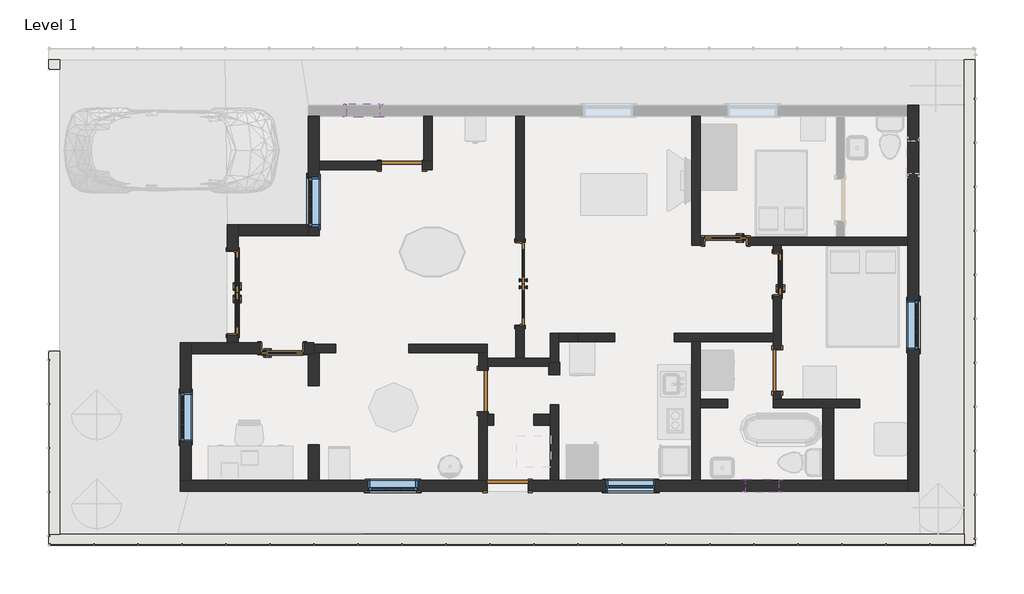
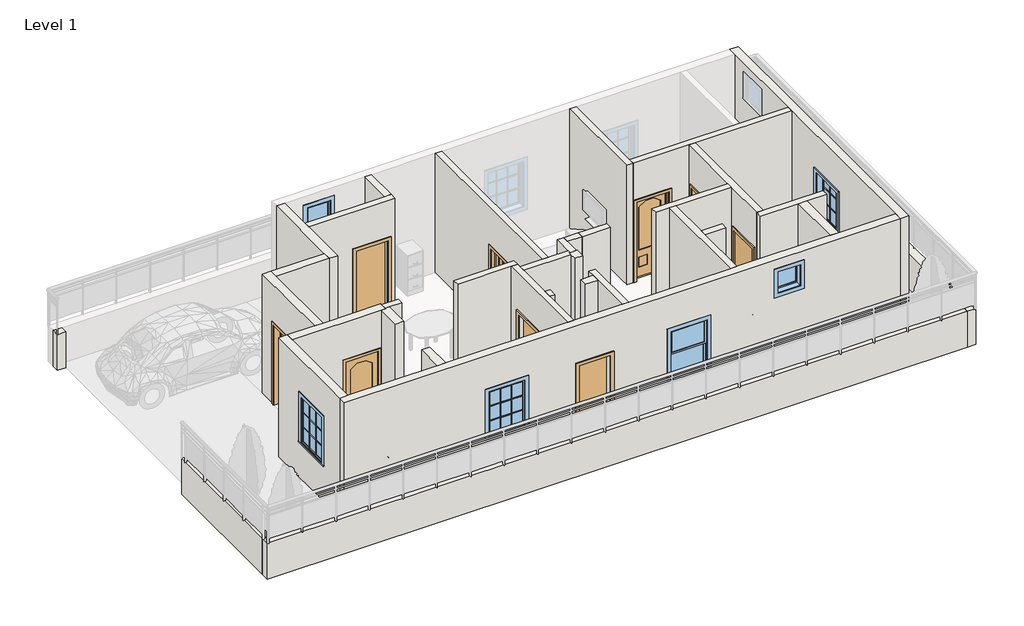
# One storey, part 1 of 3: 35 walls, 9 doors, 7 windows.
"""IFC4 building model written with IfcOpenShell, lengths in millimetres."""

from ifc_helpers import new_model, si_unit, frame, origin, origin_with_axes, place, context, project, spatial, polyline, outline, extrude, faceted_brep, transform, mapped, element, save
from components import door_ad59dcae, door_14b9be53, door_b03bd389, door_31a77bde, door_059fdd7e, door_255cab33, door_53b1b562, window_29c06734, window_31198920, window_e41d21a6

model = new_model("IFC4")

# Units and contexts
model_context = context("Model", 3, world=origin())
ifc_project = project(units=[si_unit("LENGTHUNIT", "METRE", prefix="MILLI")], contexts=[model_context])

# Site, building, storey
site = spatial("IfcSite", under=ifc_project)
building = spatial("IfcBuilding", under=site)
storey = spatial("IfcBuildingStorey", under=building, Name="Level 1", Elevation=0.0)

# Doors
placement = place(None, origin())
door_shape = door_ad59dcae(model_context)
element("IfcDoor", 1, ObjectType="30\" x 80\"", at=placement, inside=storey, context=model_context, shape_type="MappedRepresentation", body=[
    mapped(door_shape, transform((-17787.0845566, 6835.9062219, 0.0), x_axis=(-1.0, 0.0, 0.0), y_axis=(0.0, -1.0, 0.0), z_axis=(0.0, 0.0, 1.0))),
])
door_2_shape = door_14b9be53(model_context)
element("IfcDoor", 2, ObjectType="30\" x 80\"", at=placement, inside=storey, context=model_context, shape_type="MappedRepresentation", body=[
    mapped(door_2_shape, transform((-8639.9095566, 8210.6812219, 0.0), x_axis=(0.0, -1.0, 0.0), y_axis=(1.0, 0.0, 0.0), z_axis=(0.0, 0.0, 1.0))),
])
element("IfcDoor", 3, ObjectType="30\" x 80\"", at=placement, inside=storey, context=model_context, shape_type="MappedRepresentation", body=[
    mapped(door_2_shape, transform((-9595.5845566, 8823.4562219, 0.0), x_axis=(1.0, 0.0, 0.0), y_axis=(0.0, 1.0, 0.0), z_axis=(0.0, 0.0, 1.0))),
])
door_3_shape = door_b03bd389(model_context)
element("IfcDoor", 4, ObjectType="Door-Exterior-Double-Full Glass-Wood_Clad : 60\" x 80\"", at=placement, inside=storey, context=model_context, shape_type="MappedRepresentation", body=[
    mapped(door_3_shape, transform((-18698.3095566, 7867.7812219, 0.0), x_axis=(0.0, -1.0, 0.0), y_axis=(1.0, 0.0, 0.0), z_axis=(0.0, 0.0, 1.0))),
])
door_4_shape = door_31a77bde(model_context)
element("IfcDoor", 5, ObjectType="Door-Interior-Double-Full Glass-Wood : 60\" x 80\"", at=placement, inside=storey, context=model_context, shape_type="MappedRepresentation", body=[
    mapped(door_4_shape, transform((-13389.7095566, 8032.8812219, 0.0), x_axis=(0.0, -1.0, 0.0), y_axis=(1.0, 0.0, 0.0), z_axis=(0.0, 0.0, 1.0))),
])
door_5_shape = door_059fdd7e(model_context)
element("IfcDoor", 6, ObjectType="Single-Flush : 30\" x 80\"", at=placement, inside=storey, context=model_context, shape_type="MappedRepresentation", body=[
    mapped(door_5_shape, transform((-15577.2845566, 10217.2812219, 0.0), x_axis=(1.0, 0.0, 0.0), y_axis=(0.0, 1.0, 0.0), z_axis=(0.0, 0.0, 1.0))),
])
element("IfcDoor", 7, ObjectType="Single-Flush : 30\" x 80\"", at=placement, inside=storey, context=model_context, shape_type="MappedRepresentation", body=[
    mapped(door_5_shape, transform((-8643.0845566, 6432.6812219, 0.0), x_axis=(0.0, 1.0, 0.0), y_axis=(-1.0, 0.0, 0.0), z_axis=(0.0, 0.0, 1.0))),
])
door_6_shape = door_255cab33(model_context)
element("IfcDoor", 8, ObjectType="Single-Flush : 30\" x 80\"", at=placement, inside=storey, context=model_context, shape_type="MappedRepresentation", body=[
    mapped(door_6_shape, transform((-14078.6845566, 6051.6812219, 0.0), x_axis=(0.0, 1.0, 0.0), y_axis=(-1.0, 0.0, 0.0), z_axis=(0.0, 0.0, 1.0))),
])
door_7_shape = door_53b1b562(model_context)
element("IfcDoor", 9, ObjectType="Single-Flush : 30\" x 80\"", at=placement, inside=storey, context=model_context, shape_type="MappedRepresentation", body=[
    mapped(door_7_shape, transform((-13621.4845566, 4299.0812219, 0.0), x_axis=(-1.0, 0.0, 0.0), y_axis=(0.0, -1.0, 0.0), z_axis=(0.0, 0.0, 1.0))),
])

# Walls
element("IfcWall", 10, ObjectType="Generic - 8\"", at=placement, inside=storey, context=model_context, shape_type="Brep", body=[
    faceted_brep([(-5184.9202606, 12173.6658827, 0.0), (-5184.9202606, 3410.6658827, 0.0), (-5184.9202606, 3207.4658827, 0.0), (-5184.9202606, 3207.4658827, 914.4), (-5184.9202606, 3410.6658827, 914.4), (-5184.9202606, 12173.6658827, 914.4), (-4981.7202606, 12173.6658827, 0.0), (-4981.7202606, 12173.6658827, 914.4), (-4981.7202606, 3207.4658827, 914.4), (-4981.7202606, 3207.4658827, 0.0)], [[[0, 1, 2, 3, 4, 5]], [[6, 7, 8, 9]], [[2, 1, 0, 6, 9]], [[5, 4, 3, 8, 7]], [[0, 5, 7, 6]], [[3, 2, 9, 8]]]),
])
element("IfcWall", 11, ObjectType="Generic - 8\"", at=placement, inside=storey, context=model_context, shape_type="Brep", body=[
    faceted_brep([(-5184.9202606, 3410.6658827, 0.0), (-21898.1202606, 3410.6658827, 0.0), (-22101.3202606, 3410.6658827, 0.0), (-22101.3202606, 3410.6658827, 914.4), (-21898.1202606, 3410.6658827, 914.4), (-5184.9202606, 3410.6658827, 914.4), (-5184.9202606, 3207.4658827, 0.0), (-5184.9202606, 3207.4658827, 914.4), (-22101.3202606, 3207.4658827, 914.4), (-22101.3202606, 3207.4658827, 0.0)], [[[0, 1, 2, 3, 4, 5]], [[6, 7, 8, 9]], [[2, 1, 0, 6, 9]], [[5, 4, 3, 8, 7]], [[0, 5, 7, 6]], [[3, 2, 9, 8]]]),
])
element("IfcWall", 12, ObjectType="Generic - 8\"", at=placement, inside=storey, context=model_context, shape_type="SweptSolid", body=[
    extrude(outline(polyline([(-21898.1202606, 6788.8658827), (-21898.1202606, 3410.6658827), (-22101.3202606, 3410.6658827), (-22101.3202606, 6788.8658827), (-21898.1202606, 6788.8658827)])), origin_with_axes(), (0.0, 0.0, 1.0), 914.4),
])
element("IfcWall", 13, ObjectType="Generic - 8\"", at=placement, inside=storey, context=model_context, shape_type="Brep", body=[
    faceted_brep([(-6230.0845566, 11334.8812219, 0.0), (-6230.0845566, 11131.6812219, 0.0), (-6230.0845566, 8896.4812219, 0.0), (-6230.0845566, 8744.0812219, 0.0), (-6230.0845566, 4400.6812219, 0.0), (-6230.0845566, 4197.4812219, 0.0), (-6230.0845566, 4197.4812219, 3048.0), (-6230.0845566, 4400.6812219, 3048.0), (-6230.0845566, 8744.0812219, 3048.0), (-6230.0845566, 8896.4812219, 3048.0), (-6230.0845566, 11131.6812219, 3048.0), (-6230.0845566, 11334.8812219, 3048.0), (-6230.0845566, 6813.6812219, 2133.6), (-6230.0845566, 6813.6812219, 914.4), (-6230.0845566, 7728.0812219, 914.4), (-6230.0845566, 7728.0812219, 2133.6), (-6230.0845566, 10674.4812219, 2768.6), (-6230.0845566, 10064.8812219, 2768.6), (-6230.0845566, 10064.8812219, 2159.0), (-6230.0845566, 10674.4812219, 2159.0), (-6026.8845566, 11334.8812219, 0.0), (-6026.8845566, 11334.8812219, 3048.0), (-6026.8845566, 4197.4812219, 3048.0), (-6026.8845566, 4197.4812219, 0.0), (-6026.8845566, 6813.6812219, 2133.6), (-6026.8845566, 7728.0812219, 2133.6), (-6026.8845566, 7728.0812219, 914.4), (-6026.8845566, 6813.6812219, 914.4), (-6026.8845566, 10674.4812219, 2768.6), (-6026.8845566, 10674.4812219, 2159.0), (-6026.8845566, 10064.8812219, 2159.0), (-6026.8845566, 10064.8812219, 2768.6)], [[[0, 1, 2, 3, 4, 5, 6, 7, 8, 9, 10, 11], [12, 13, 14, 15], [16, 17, 18, 19]], [[20, 21, 22, 23], [24, 25, 26, 27], [28, 29, 30, 31]], [[5, 4, 3, 2, 1, 0, 20, 23]], [[6, 5, 23, 22]], [[0, 11, 21, 20]], [[11, 10, 9, 8, 7, 6, 22, 21]], [[13, 12, 24, 27]], [[14, 13, 27, 26]], [[15, 14, 26, 25]], [[12, 15, 25, 24]], [[29, 28, 16, 19]], [[30, 29, 19, 18]], [[31, 30, 18, 17]], [[28, 31, 17, 16]]]),
])
element("IfcWall", 14, ObjectType="Generic - 8\"", at=placement, inside=storey, context=model_context, shape_type="Brep", body=[
    faceted_brep([(-14002.4845566, 4400.6812219, 2032.0), (-14002.4845566, 4400.6812219, 0.0), (-14154.8845566, 4400.6812219, 0.0), (-17101.2845566, 4400.6812219, 0.0), (-17304.4845566, 4400.6812219, 0.0), (-19463.4845566, 4400.6812219, 0.0), (-19666.6845566, 4400.6812219, 0.0), (-19666.6845566, 4400.6812219, 3048.0), (-19463.4845566, 4400.6812219, 3048.0), (-17304.4845566, 4400.6812219, 3048.0), (-17101.2845566, 4400.6812219, 3048.0), (-14154.8845566, 4400.6812219, 3048.0), (-14002.4845566, 4400.6812219, 3048.0), (-12834.0845566, 4400.6812219, 3048.0), (-12681.6845566, 4400.6812219, 3048.0), (-10217.8845566, 4400.6812219, 3048.0), (-10065.4845566, 4400.6812219, 3048.0), (-7804.8845566, 4400.6812219, 3048.0), (-7601.6845566, 4400.6812219, 3048.0), (-6230.0845566, 4400.6812219, 3048.0), (-6230.0845566, 4400.6812219, 0.0), (-7601.6845566, 4400.6812219, 0.0), (-7804.8845566, 4400.6812219, 0.0), (-10065.4845566, 4400.6812219, 0.0), (-10217.8845566, 4400.6812219, 0.0), (-12681.6845566, 4400.6812219, 0.0), (-12834.0845566, 4400.6812219, 0.0), (-13240.4845566, 4400.6812219, 0.0), (-13240.4845566, 4400.6812219, 2032.0), (-16199.5845566, 4400.6812219, 2133.6), (-16199.5845566, 4400.6812219, 914.4), (-15285.1845566, 4400.6812219, 914.4), (-15285.1845566, 4400.6812219, 2133.6), (-11805.3845566, 4400.6812219, 2133.6), (-11805.3845566, 4400.6812219, 914.4), (-10890.9845566, 4400.6812219, 914.4), (-10890.9845566, 4400.6812219, 2133.6), (-8617.6845566, 4400.6812219, 2768.6), (-9227.2845566, 4400.6812219, 2768.6), (-9227.2845566, 4400.6812219, 2159.0), (-8617.6845566, 4400.6812219, 2159.0), (-19666.6845566, 4197.4812219, 0.0), (-14002.4845566, 4197.4812219, 0.0), (-14002.4845566, 4197.4812219, 2032.0), (-13240.4845566, 4197.4812219, 2032.0), (-13240.4845566, 4197.4812219, 0.0), (-6230.0845566, 4197.4812219, 0.0), (-6230.0845566, 4197.4812219, 3048.0), (-19666.6845566, 4197.4812219, 3048.0), (-16199.5845566, 4197.4812219, 2133.6), (-15285.1845566, 4197.4812219, 2133.6), (-15285.1845566, 4197.4812219, 914.4), (-16199.5845566, 4197.4812219, 914.4), (-11805.3845566, 4197.4812219, 2133.6), (-10890.9845566, 4197.4812219, 2133.6), (-10890.9845566, 4197.4812219, 914.4), (-11805.3845566, 4197.4812219, 914.4), (-8617.6845566, 4197.4812219, 2768.6), (-8617.6845566, 4197.4812219, 2159.0), (-9227.2845566, 4197.4812219, 2159.0), (-9227.2845566, 4197.4812219, 2768.6)], [[[0, 1, 2, 3, 4, 5, 6, 7, 8, 9, 10, 11, 12, 13, 14, 15, 16, 17, 18, 19, 20, 21, 22, 23, 24, 25, 26, 27, 28], [29, 30, 31, 32], [33, 34, 35, 36], [37, 38, 39, 40]], [[41, 42, 43, 44, 45, 46, 47, 48], [49, 50, 51, 52], [53, 54, 55, 56], [57, 58, 59, 60]], [[6, 5, 4, 3, 2, 1, 42, 41]], [[27, 26, 25, 24, 23, 22, 21, 20, 46, 45]], [[20, 19, 47, 46]], [[7, 6, 41, 48]], [[43, 42, 1, 0]], [[44, 43, 0, 28]], [[45, 44, 28, 27]], [[19, 18, 17, 16, 15, 14, 13, 12, 11, 10, 9, 8, 7, 48, 47]], [[30, 29, 49, 52]], [[31, 30, 52, 51]], [[32, 31, 51, 50]], [[29, 32, 50, 49]], [[34, 33, 53, 56]], [[35, 34, 56, 55]], [[36, 35, 55, 54]], [[33, 36, 54, 53]], [[58, 57, 37, 40]], [[59, 58, 40, 39]], [[60, 59, 39, 38]], [[57, 60, 38, 37]]]),
])
element("IfcWall", 15, ObjectType="Generic - 8\"", at=placement, inside=storey, context=model_context, shape_type="Brep", body=[
    faceted_brep([(-19463.4845566, 4400.6812219, 0.0), (-19463.4845566, 6737.4812219, 0.0), (-19463.4845566, 6940.6812219, 0.0), (-19463.4845566, 6940.6812219, 3048.0), (-19463.4845566, 6737.4812219, 3048.0), (-19463.4845566, 4400.6812219, 3048.0), (-19463.4845566, 6026.2812219, 2133.6), (-19463.4845566, 6026.2812219, 914.4), (-19463.4845566, 5111.8812219, 914.4), (-19463.4845566, 5111.8812219, 2133.6), (-19666.6845566, 4400.6812219, 0.0), (-19666.6845566, 4400.6812219, 3048.0), (-19666.6845566, 6940.6812219, 3048.0), (-19666.6845566, 6940.6812219, 0.0), (-19666.6845566, 6026.2812219, 2133.6), (-19666.6845566, 5111.8812219, 2133.6), (-19666.6845566, 5111.8812219, 914.4), (-19666.6845566, 6026.2812219, 914.4)], [[[0, 1, 2, 3, 4, 5], [6, 7, 8, 9]], [[10, 11, 12, 13], [14, 15, 16, 17]], [[2, 1, 0, 10, 13]], [[0, 5, 11, 10]], [[3, 2, 13, 12]], [[5, 4, 3, 12, 11]], [[7, 6, 14, 17]], [[8, 7, 17, 16]], [[9, 8, 16, 15]], [[6, 9, 15, 14]]]),
])
element("IfcWall", 16, ObjectType="Generic - 8\"", at=placement, inside=storey, context=model_context, shape_type="Brep", body=[
    faceted_brep([(-17202.8845566, 6737.4812219, 0.0), (-17202.8845566, 6737.4812219, 3048.0), (-17304.4845566, 6737.4812219, 3048.0), (-19463.4845566, 6737.4812219, 3048.0), (-19463.4845566, 6737.4812219, 0.0), (-18193.4845566, 6737.4812219, 0.0), (-18193.4845566, 6737.4812219, 2057.4), (-17380.6845566, 6737.4812219, 2057.4), (-17380.6845566, 6737.4812219, 0.0), (-17304.4845566, 6737.4812219, 0.0), (-17202.8845566, 6940.6812219, 3048.0), (-17202.8845566, 6940.6812219, 0.0), (-17380.6845566, 6940.6812219, 0.0), (-17380.6845566, 6940.6812219, 2057.4), (-18193.4845566, 6940.6812219, 2057.4), (-18193.4845566, 6940.6812219, 0.0), (-18599.8845566, 6940.6812219, 0.0), (-18803.0845566, 6940.6812219, 0.0), (-19463.4845566, 6940.6812219, 0.0), (-19463.4845566, 6940.6812219, 3048.0), (-18803.0845566, 6940.6812219, 3048.0), (-18599.8845566, 6940.6812219, 3048.0), (-17202.8845566, 6915.2812219, 0.0), (-17202.8845566, 6762.8812219, 0.0), (-17202.8845566, 6915.2812219, 3048.0), (-17202.8845566, 6762.8812219, 3048.0)], [[[0, 1, 2, 3, 4, 5, 6, 7, 8, 9]], [[10, 11, 12, 13, 14, 15, 16, 17, 18, 19, 20, 21]], [[4, 18, 17, 16, 15, 5]], [[11, 22, 23, 0, 9, 8, 12]], [[1, 0, 23, 22, 11, 10, 24, 25]], [[4, 3, 19, 18]], [[14, 6, 5, 15]], [[6, 14, 13, 7]], [[7, 13, 12, 8]], [[3, 2, 1, 25, 24, 10, 21, 20, 19]]]),
])
element("IfcWall", 17, ObjectType="Generic - 8\"", at=placement, inside=storey, context=model_context, shape_type="Brep", body=[
    faceted_brep([(-17304.4845566, 11131.6812219, 0.0), (-17304.4845566, 9125.0812219, 0.0), (-17304.4845566, 8921.8812219, 0.0), (-17304.4845566, 8921.8812219, 3048.0), (-17304.4845566, 9125.0812219, 3048.0), (-17304.4845566, 11131.6812219, 3048.0), (-17304.4845566, 10001.3812219, 2133.6), (-17304.4845566, 9086.9812219, 2133.6), (-17304.4845566, 9086.9812219, 914.4), (-17304.4845566, 10001.3812219, 914.4), (-17101.2845566, 11131.6812219, 0.0), (-17101.2845566, 11131.6812219, 3048.0), (-17101.2845566, 10293.4812219, 3048.0), (-17101.2845566, 10141.0812219, 3048.0), (-17101.2845566, 8921.8812219, 3048.0), (-17101.2845566, 8921.8812219, 0.0), (-17101.2845566, 10141.0812219, 0.0), (-17101.2845566, 10293.4812219, 0.0), (-17101.2845566, 10001.3812219, 2133.6), (-17101.2845566, 10001.3812219, 914.4), (-17101.2845566, 9086.9812219, 914.4), (-17101.2845566, 9086.9812219, 2133.6)], [[[0, 1, 2, 3, 4, 5], [6, 7, 8, 9]], [[10, 11, 12, 13, 14, 15, 16, 17], [18, 19, 20, 21]], [[2, 1, 0, 10, 17, 16, 15]], [[0, 5, 11, 10]], [[3, 2, 15, 14]], [[5, 4, 3, 14, 13, 12, 11]], [[19, 18, 6, 9]], [[20, 19, 9, 8]], [[21, 20, 8, 7]], [[18, 21, 7, 6]]]),
])
element("IfcWall", 18, ObjectType="Generic - 8\"", at=placement, inside=storey, context=model_context, shape_type="Brep", body=[
    faceted_brep([(-18599.8845566, 6940.6812219, 3048.0), (-18599.8845566, 6940.6812219, 0.0), (-18599.8845566, 7080.3812219, 0.0), (-18599.8845566, 7080.3812219, 2057.4), (-18599.8845566, 8655.1812219, 2057.4), (-18599.8845566, 8655.1812219, 0.0), (-18599.8845566, 8921.8812219, 0.0), (-18599.8845566, 9125.0812219, 0.0), (-18599.8845566, 9125.0812219, 3048.0), (-18599.8845566, 8921.8812219, 3048.0), (-18803.0845566, 6940.6812219, 0.0), (-18803.0845566, 6940.6812219, 3048.0), (-18803.0845566, 9125.0812219, 3048.0), (-18803.0845566, 9125.0812219, 0.0), (-18803.0845566, 8655.1812219, 0.0), (-18803.0845566, 8655.1812219, 2057.4), (-18803.0845566, 7080.3812219, 2057.4), (-18803.0845566, 7080.3812219, 0.0)], [[[0, 1, 2, 3, 4, 5, 6, 7, 8, 9]], [[10, 11, 12, 13, 14, 15, 16, 17]], [[1, 10, 17, 2]], [[13, 7, 6, 5, 14]], [[1, 0, 11, 10]], [[8, 7, 13, 12]], [[16, 3, 2, 17]], [[3, 16, 15, 4]], [[4, 15, 14, 5]], [[0, 9, 8, 12, 11]]]),
])
element("IfcWall", 19, ObjectType="Generic - 8\"", at=placement, inside=storey, context=model_context, shape_type="SweptSolid", body=[
    extrude(outline(polyline([(-17304.4845566, 8921.8812219), (-18599.8845566, 8921.8812219), (-18599.8845566, 9125.0812219), (-17304.4845566, 9125.0812219), (-17304.4845566, 8921.8812219)])), origin_with_axes(), (0.0, 0.0, 1.0), 3048.0),
])
element("IfcWall", 20, ObjectType="Generic - 8\"", at=placement, inside=storey, context=model_context, shape_type="SweptSolid", body=[
    extrude(outline(polyline([(-17304.4845566, 4400.6812219), (-17304.4845566, 5061.0812219), (-17101.2845566, 5061.0812219), (-17101.2845566, 4400.6812219), (-17304.4845566, 4400.6812219)])), origin_with_axes(), (0.0, 0.0, 1.0), 3048.0),
])
element("IfcWall", 21, ObjectType="Generic - 8\"", at=placement, inside=storey, context=model_context, shape_type="SweptSolid", body=[
    extrude(outline(polyline([(-17304.4845566, 6153.2812219), (-17304.4845566, 6737.4812219), (-17202.8845566, 6737.4812219), (-17202.8845566, 6762.8812219), (-17101.2845566, 6762.8812219), (-17101.2845566, 6153.2812219), (-17304.4845566, 6153.2812219)])), origin_with_axes(), (0.0, 0.0, 1.0), 3048.0),
])
element("IfcWall", 22, ObjectType="Generic - 8\"", at=placement, inside=storey, context=model_context, shape_type="SweptSolid", body=[
    extrude(outline(polyline([(-7804.8845566, 4400.6812219), (-7804.8845566, 5746.8812219), (-7601.6845566, 5746.8812219), (-7601.6845566, 4400.6812219), (-7804.8845566, 4400.6812219)])), origin_with_axes(), (0.0, 0.0, 1.0), 3048.0),
])
element("IfcWall", 23, ObjectType="Generic - 8\"", at=placement, inside=storey, context=model_context, shape_type="SweptSolid", body=[
    extrude(outline(polyline([(-21898.1202606, 12173.6658827), (-21898.1202606, 11995.8658827), (-22101.3202606, 11995.8658827), (-22101.3202606, 12173.6658827), (-21898.1202606, 12173.6658827)])), origin_with_axes(), (0.0, 0.0, 1.0), 914.4),
])
element("IfcWall", 24, ObjectType="Generic - 8\"", at=placement, inside=storey, context=model_context, shape_type="SweptSolid", body=[
    extrude(outline(polyline([(-13138.8845566, 5619.8812219), (-12834.0845566, 5619.8812219), (-12834.0845566, 5416.6812219), (-13138.8845566, 5416.6812219), (-13138.8845566, 5619.8812219)])), origin_with_axes(), (0.0, 0.0, 1.0), 3048.0),
])
element("IfcWall", 25, ObjectType="Generic - 8\"", at=placement, inside=storey, context=model_context, shape_type="SweptSolid", body=[
    extrude(outline(polyline([(-14002.4845566, 5619.8812219), (-13875.4845566, 5619.8812219), (-13875.4845566, 5416.6812219), (-14002.4845566, 5416.6812219), (-14002.4845566, 5619.8812219)])), origin_with_axes(), (0.0, 0.0, 1.0), 3048.0),
])
element("IfcWall", 26, ObjectType="Generic - 8\"", at=placement, inside=storey, context=model_context, shape_type="Brep", body=[
    faceted_brep([(-12859.4845566, 6585.0812219, 0.0), (-12859.4845566, 6508.8812219, 0.0), (-12859.4845566, 6356.4812219, 0.0), (-12859.4845566, 6356.4812219, 3048.0), (-12859.4845566, 6508.8812219, 3048.0), (-12859.4845566, 6585.0812219, 3048.0), (-12656.2845566, 6585.0812219, 0.0), (-12656.2845566, 6585.0812219, 3048.0), (-12656.2845566, 6356.4812219, 3048.0), (-12656.2845566, 6356.4812219, 0.0), (-12834.0845566, 6585.0812219, 0.0), (-12681.6845566, 6585.0812219, 0.0), (-12681.6845566, 6585.0812219, 3048.0), (-12834.0845566, 6585.0812219, 3048.0)], [[[0, 1, 2, 3, 4, 5]], [[6, 7, 8, 9]], [[2, 1, 0, 10, 11, 6, 9]], [[3, 2, 9, 8]], [[5, 4, 3, 8, 7, 12, 13]], [[0, 5, 13, 12, 7, 6, 11, 10]]]),
])
element("IfcWall", 27, ObjectType="INNER WALL", at=placement, inside=storey, context=model_context, shape_type="Brep", body=[
    faceted_brep([(-15196.2845566, 10141.0812219, 2032.0), (-15196.2845566, 10141.0812219, 0.0), (-15018.4845566, 10141.0812219, 0.0), (-15018.4845566, 10141.0812219, 3048.0), (-17101.2845566, 10141.0812219, 3048.0), (-17101.2845566, 10141.0812219, 0.0), (-15958.2845566, 10141.0812219, 0.0), (-15958.2845566, 10141.0812219, 2032.0), (-15018.4845566, 10293.4812219, 0.0), (-15170.8845566, 10293.4812219, 0.0), (-15196.2845566, 10293.4812219, 0.0), (-15196.2845566, 10293.4812219, 2032.0), (-15958.2845566, 10293.4812219, 2032.0), (-15958.2845566, 10293.4812219, 0.0), (-17101.2845566, 10293.4812219, 0.0), (-17101.2845566, 10293.4812219, 3048.0), (-15170.8845566, 10293.4812219, 3048.0), (-15018.4845566, 10293.4812219, 3048.0)], [[[0, 1, 2, 3, 4, 5, 6, 7]], [[8, 9, 10, 11, 12, 13, 14, 15, 16, 17]], [[6, 5, 14, 13]], [[2, 1, 10, 9, 8]], [[5, 4, 15, 14]], [[3, 2, 8, 17]], [[11, 10, 1, 0]], [[12, 11, 0, 7]], [[13, 12, 7, 6]], [[4, 3, 17, 16, 15]]]),
])
element("IfcWall", 28, ObjectType="INNER WALL", at=placement, inside=storey, context=model_context, shape_type="SweptSolid", body=[
    extrude(outline(polyline([(-15018.4845566, 11131.6812219), (-15018.4845566, 10293.4812219), (-15170.8845566, 10293.4812219), (-15170.8845566, 11131.6812219), (-15018.4845566, 11131.6812219)])), origin_with_axes(), (0.0, 0.0, 1.0), 3048.0),
])
element("IfcWall", 29, ObjectType="INNER WALL", at=placement, inside=storey, context=model_context, shape_type="SweptSolid", body=[
    extrude(outline(polyline([(11131.6812219, 3048.0), (11131.6812219, 0.0), (8820.2812219, 0.0), (8820.2812219, 2057.4), (7245.4812219, 2057.4), (7245.4812219, 0.0), (6661.2812219, 0.0), (6661.2812219, 3048.0), (11131.6812219, 3048.0)])), frame((-13469.0845566, 0.0, 0.0), z_axis=(1.0, 0.0, 0.0), x_axis=(0.0, 1.0, 0.0)), (0.0, 0.0, 1.0), 152.4),
])
element("IfcWall", 30, ObjectType="INNER WALL", at=placement, inside=storey, context=model_context, shape_type="Brep", body=[
    faceted_brep([(-17202.8845566, 6762.8812219, 0.0), (-17101.2845566, 6762.8812219, 0.0), (-16796.4845566, 6762.8812219, 0.0), (-16796.4845566, 6762.8812219, 3048.0), (-17101.2845566, 6762.8812219, 3048.0), (-17202.8845566, 6762.8812219, 3048.0), (-17202.8845566, 6915.2812219, 0.0), (-17202.8845566, 6915.2812219, 3048.0), (-16796.4845566, 6915.2812219, 3048.0), (-16796.4845566, 6915.2812219, 0.0)], [[[0, 1, 2, 3, 4, 5]], [[6, 7, 8, 9]], [[2, 1, 0, 6, 9]], [[3, 2, 9, 8]], [[0, 5, 7, 6]], [[5, 4, 3, 8, 7]]]),
])
element("IfcWall", 31, ObjectType="INNER WALL", at=placement, inside=storey, context=model_context, shape_type="Brep", body=[
    faceted_brep([(-14154.8845566, 6762.8812219, 0.0), (-14154.8845566, 6432.6812219, 0.0), (-14154.8845566, 6432.6812219, 2032.0), (-14154.8845566, 5670.6812219, 2032.0), (-14154.8845566, 5670.6812219, 0.0), (-14154.8845566, 4400.6812219, 0.0), (-14154.8845566, 4400.6812219, 3048.0), (-14154.8845566, 6762.8812219, 3048.0), (-14002.4845566, 6432.6812219, 2032.0), (-14002.4845566, 6432.6812219, 0.0), (-14002.4845566, 6508.8812219, 0.0), (-14002.4845566, 6661.2812219, 0.0), (-14002.4845566, 6762.8812219, 0.0), (-14002.4845566, 6762.8812219, 3048.0), (-14002.4845566, 6661.2812219, 3048.0), (-14002.4845566, 6508.8812219, 3048.0), (-14002.4845566, 5619.8812219, 3048.0), (-14002.4845566, 5416.6812219, 3048.0), (-14002.4845566, 4400.6812219, 3048.0), (-14002.4845566, 4400.6812219, 2032.0), (-14002.4845566, 4400.6812219, 0.0), (-14002.4845566, 5416.6812219, 0.0), (-14002.4845566, 5619.8812219, 0.0), (-14002.4845566, 5670.6812219, 0.0), (-14002.4845566, 5670.6812219, 2032.0)], [[[0, 1, 2, 3, 4, 5, 6, 7]], [[8, 9, 10, 11, 12, 13, 14, 15, 16, 17, 18, 19, 20, 21, 22, 23, 24]], [[12, 11, 10, 9, 1, 0]], [[23, 22, 21, 20, 5, 4]], [[0, 7, 13, 12]], [[6, 5, 20, 19, 18]], [[2, 1, 9, 8]], [[3, 2, 8, 24]], [[4, 3, 24, 23]], [[7, 6, 18, 17, 16, 15, 14, 13]]]),
])
element("IfcWall", 32, ObjectType="INNER WALL", at=placement, inside=storey, context=model_context, shape_type="Brep", body=[
    faceted_brep([(-14002.4845566, 6508.8812219, 0.0), (-12859.4845566, 6508.8812219, 0.0), (-12859.4845566, 6508.8812219, 3048.0), (-14002.4845566, 6508.8812219, 3048.0), (-14002.4845566, 6661.2812219, 0.0), (-14002.4845566, 6661.2812219, 3048.0), (-13469.0845566, 6661.2812219, 3048.0), (-13316.6845566, 6661.2812219, 3048.0), (-12834.0845566, 6661.2812219, 3048.0), (-12834.0845566, 6661.2812219, 0.0), (-13316.6845566, 6661.2812219, 0.0), (-13469.0845566, 6661.2812219, 0.0), (-12834.0845566, 6585.0812219, 0.0), (-12859.4845566, 6585.0812219, 0.0), (-12859.4845566, 6585.0812219, 3048.0), (-12834.0845566, 6585.0812219, 3048.0)], [[[0, 1, 2, 3]], [[4, 5, 6, 7, 8, 9, 10, 11]], [[1, 0, 4, 11, 10, 9, 12, 13]], [[0, 3, 5, 4]], [[3, 2, 14, 15, 8, 7, 6, 5]], [[2, 1, 13, 14]], [[13, 12, 15, 14]], [[12, 9, 8, 15]]]),
])
element("IfcWall", 33, ObjectType="INNER WALL", at=placement, inside=storey, context=model_context, shape_type="Brep", body=[
    faceted_brep([(-12681.6845566, 4400.6812219, 0.0), (-12681.6845566, 5797.6812219, 0.0), (-12681.6845566, 5797.6812219, 3048.0), (-12681.6845566, 4400.6812219, 3048.0), (-12834.0845566, 4400.6812219, 0.0), (-12834.0845566, 4400.6812219, 3048.0), (-12834.0845566, 5416.6812219, 3048.0), (-12834.0845566, 5619.8812219, 3048.0), (-12834.0845566, 5797.6812219, 3048.0), (-12834.0845566, 5797.6812219, 0.0), (-12834.0845566, 5619.8812219, 0.0), (-12834.0845566, 5416.6812219, 0.0)], [[[0, 1, 2, 3]], [[4, 5, 6, 7, 8, 9, 10, 11]], [[1, 0, 4, 11, 10, 9]], [[2, 1, 9, 8]], [[0, 3, 5, 4]], [[3, 2, 8, 7, 6, 5]]]),
])
element("IfcWall", 34, ObjectType="INNER WALL", at=placement, inside=storey, context=model_context, shape_type="SweptSolid", body=[
    extrude(outline(polyline([(-12326.0845566, 6966.0812219), (-12681.6845566, 6966.0812219), (-12681.6845566, 7118.4812219), (-12326.0845566, 7118.4812219), (-12326.0845566, 6966.0812219)])), origin_with_axes(), (0.0, 0.0, 1.0), 3048.0),
])
element("IfcWall", 35, ObjectType="INNER WALL", at=placement, inside=storey, context=model_context, shape_type="Brep", body=[
    faceted_brep([(-8719.2845566, 7804.2812219, 0.0), (-8719.2845566, 7118.4812219, 0.0), (-8719.2845566, 6966.0812219, 0.0), (-8719.2845566, 6813.6812219, 0.0), (-8719.2845566, 6813.6812219, 2032.0), (-8719.2845566, 6051.6812219, 2032.0), (-8719.2845566, 6051.6812219, 0.0), (-8719.2845566, 5899.2812219, 0.0), (-8719.2845566, 5899.2812219, 3048.0), (-8719.2845566, 6966.0812219, 3048.0), (-8719.2845566, 7118.4812219, 3048.0), (-8719.2845566, 8744.0812219, 3048.0), (-8719.2845566, 8744.0812219, 0.0), (-8719.2845566, 8617.0812219, 0.0), (-8719.2845566, 8617.0812219, 2057.4), (-8719.2845566, 7804.2812219, 2057.4), (-8566.8845566, 6813.6812219, 2032.0), (-8566.8845566, 6813.6812219, 0.0), (-8566.8845566, 7804.2812219, 0.0), (-8566.8845566, 7804.2812219, 2057.4), (-8566.8845566, 8617.0812219, 2057.4), (-8566.8845566, 8617.0812219, 0.0), (-8566.8845566, 8744.0812219, 0.0), (-8566.8845566, 8744.0812219, 3048.0), (-8566.8845566, 5899.2812219, 3048.0), (-8566.8845566, 5899.2812219, 0.0), (-8566.8845566, 6051.6812219, 0.0), (-8566.8845566, 6051.6812219, 2032.0)], [[[0, 1, 2, 3, 4, 5, 6, 7, 8, 9, 10, 11, 12, 13, 14, 15]], [[16, 17, 18, 19, 20, 21, 22, 23, 24, 25, 26, 27]], [[12, 22, 21, 13]], [[26, 25, 7, 6]], [[18, 17, 3, 2, 1, 0]], [[12, 11, 23, 22]], [[8, 7, 25, 24]], [[15, 19, 18, 0]], [[19, 15, 14, 20]], [[20, 14, 13, 21]], [[11, 10, 9, 8, 24, 23]], [[4, 3, 17, 16]], [[5, 4, 16, 27]], [[6, 5, 27, 26]]]),
])
element("IfcWall", 36, ObjectType="INNER WALL", at=placement, inside=storey, context=model_context, shape_type="SweptSolid", body=[
    extrude(outline(polyline([(-9557.4845566, 5746.8812219), (-10065.4845566, 5746.8812219), (-10065.4845566, 5899.2812219), (-9557.4845566, 5899.2812219), (-9557.4845566, 5746.8812219)])), origin_with_axes(), (0.0, 0.0, 1.0), 3048.0),
])
element("IfcWall", 37, ObjectType="INNER WALL", at=placement, inside=storey, context=model_context, shape_type="Brep", body=[
    faceted_brep([(-10217.8845566, 11131.6812219, 0.0), (-10217.8845566, 8744.0812219, 0.0), (-10217.8845566, 8744.0812219, 3048.0), (-10217.8845566, 11131.6812219, 3048.0), (-10065.4845566, 11131.6812219, 0.0), (-10065.4845566, 11131.6812219, 3048.0), (-10065.4845566, 8896.4812219, 3048.0), (-10065.4845566, 8744.0812219, 3048.0), (-10065.4845566, 8744.0812219, 0.0), (-10065.4845566, 8896.4812219, 0.0)], [[[0, 1, 2, 3]], [[4, 5, 6, 7, 8, 9]], [[1, 0, 4, 9, 8]], [[0, 3, 5, 4]], [[2, 1, 8, 7]], [[3, 2, 7, 6, 5]]]),
])
element("IfcWall", 38, ObjectType="INNER WALL", at=placement, inside=storey, context=model_context, shape_type="Brep", body=[
    faceted_brep([(-6230.0845566, 8744.0812219, 0.0), (-6230.0845566, 8744.0812219, 3048.0), (-8566.8845566, 8744.0812219, 3048.0), (-8719.2845566, 8744.0812219, 3048.0), (-10065.4845566, 8744.0812219, 3048.0), (-10065.4845566, 8744.0812219, 0.0), (-10001.9845566, 8744.0812219, 0.0), (-10001.9845566, 8744.0812219, 2057.4), (-9189.1845566, 8744.0812219, 2057.4), (-9189.1845566, 8744.0812219, 0.0), (-8719.2845566, 8744.0812219, 0.0), (-8566.8845566, 8744.0812219, 0.0), (-6230.0845566, 8896.4812219, 3048.0), (-6230.0845566, 8896.4812219, 0.0), (-7398.4845566, 8896.4812219, 0.0), (-7550.8845566, 8896.4812219, 0.0), (-9189.1845566, 8896.4812219, 0.0), (-9189.1845566, 8896.4812219, 2057.4), (-10001.9845566, 8896.4812219, 2057.4), (-10001.9845566, 8896.4812219, 0.0), (-10065.4845566, 8896.4812219, 0.0), (-10065.4845566, 8896.4812219, 3048.0), (-7550.8845566, 8896.4812219, 3048.0), (-7398.4845566, 8896.4812219, 3048.0)], [[[0, 1, 2, 3, 4, 5, 6, 7, 8, 9, 10, 11]], [[12, 13, 14, 15, 16, 17, 18, 19, 20, 21, 22, 23]], [[13, 0, 11, 10, 9, 16, 15, 14]], [[5, 20, 19, 6]], [[1, 0, 13, 12]], [[5, 4, 21, 20]], [[8, 17, 16, 9]], [[17, 8, 7, 18]], [[18, 7, 6, 19]], [[4, 3, 2, 1, 12, 23, 22, 21]]]),
])
element("IfcWall", 39, ObjectType="INNER WALL", at=placement, inside=storey, context=model_context, shape_type="Brep", body=[
    faceted_brep([(-10217.8845566, 6966.0812219, 0.0), (-10217.8845566, 4400.6812219, 0.0), (-10217.8845566, 4400.6812219, 3048.0), (-10217.8845566, 6966.0812219, 3048.0), (-10065.4845566, 6966.0812219, 0.0), (-10065.4845566, 6966.0812219, 3048.0), (-10065.4845566, 5899.2812219, 3048.0), (-10065.4845566, 5746.8812219, 3048.0), (-10065.4845566, 4400.6812219, 3048.0), (-10065.4845566, 4400.6812219, 0.0), (-10065.4845566, 5746.8812219, 0.0), (-10065.4845566, 5899.2812219, 0.0)], [[[0, 1, 2, 3]], [[4, 5, 6, 7, 8, 9, 10, 11]], [[1, 0, 4, 11, 10, 9]], [[2, 1, 9, 8]], [[0, 3, 5, 4]], [[3, 2, 8, 7, 6, 5]]]),
])
element("IfcWall", 40, ObjectType="INNER WALL", at=placement, inside=storey, context=model_context, shape_type="Brep", body=[
    faceted_brep([(-8719.2845566, 5746.8812219, 0.0), (-7804.8845566, 5746.8812219, 0.0), (-7601.6845566, 5746.8812219, 0.0), (-7119.0845566, 5746.8812219, 0.0), (-7119.0845566, 5746.8812219, 3048.0), (-7601.6845566, 5746.8812219, 3048.0), (-7804.8845566, 5746.8812219, 3048.0), (-8719.2845566, 5746.8812219, 3048.0), (-8719.2845566, 5899.2812219, 0.0), (-8719.2845566, 5899.2812219, 3048.0), (-8566.8845566, 5899.2812219, 3048.0), (-7119.0845566, 5899.2812219, 3048.0), (-7119.0845566, 5899.2812219, 0.0), (-8566.8845566, 5899.2812219, 0.0)], [[[0, 1, 2, 3, 4, 5, 6, 7]], [[8, 9, 10, 11, 12, 13]], [[3, 2, 1, 0, 8, 13, 12]], [[4, 3, 12, 11]], [[0, 7, 9, 8]], [[7, 6, 5, 4, 11, 10, 9]]]),
])
element("IfcWall", 41, ObjectType="INNER WALL", at=placement, inside=storey, context=model_context, shape_type="Brep", body=[
    faceted_brep([(-10548.0845566, 6966.0812219, 0.0), (-10217.8845566, 6966.0812219, 0.0), (-10065.4845566, 6966.0812219, 0.0), (-8719.2845566, 6966.0812219, 0.0), (-8719.2845566, 6966.0812219, 3048.0), (-10065.4845566, 6966.0812219, 3048.0), (-10217.8845566, 6966.0812219, 3048.0), (-10548.0845566, 6966.0812219, 3048.0), (-10548.0845566, 7118.4812219, 0.0), (-10548.0845566, 7118.4812219, 3048.0), (-8719.2845566, 7118.4812219, 3048.0), (-8719.2845566, 7118.4812219, 0.0)], [[[0, 1, 2, 3, 4, 5, 6, 7]], [[8, 9, 10, 11]], [[3, 2, 1, 0, 8, 11]], [[0, 7, 9, 8]], [[4, 3, 11, 10]], [[7, 6, 5, 4, 10, 9]]]),
])
element("IfcWall", 42, ObjectType="INNER WALL", at=placement, inside=storey, context=model_context, shape_type="SweptSolid", body=[
    extrude(outline(polyline([(-11640.2845566, 6966.0812219), (-12326.0845566, 6966.0812219), (-12326.0845566, 7118.4812219), (-11640.2845566, 7118.4812219), (-11640.2845566, 6966.0812219)])), origin_with_axes(), (0.0, 0.0, 1.0), 3048.0),
])
element("IfcWall", 43, ObjectType="INNER WALL", at=placement, inside=storey, context=model_context, shape_type="Brep", body=[
    faceted_brep([(-15450.2845566, 6762.8812219, 0.0), (-14154.8845566, 6762.8812219, 0.0), (-14002.4845566, 6762.8812219, 0.0), (-14002.4845566, 6762.8812219, 3048.0), (-14154.8845566, 6762.8812219, 3048.0), (-15450.2845566, 6762.8812219, 3048.0), (-15450.2845566, 6915.2812219, 0.0), (-15450.2845566, 6915.2812219, 3048.0), (-14002.4845566, 6915.2812219, 3048.0), (-14002.4845566, 6915.2812219, 0.0)], [[[0, 1, 2, 3, 4, 5]], [[6, 7, 8, 9]], [[2, 1, 0, 6, 9]], [[0, 5, 7, 6]], [[3, 2, 9, 8]], [[5, 4, 3, 8, 7]]]),
])
element("IfcWall", 44, ObjectType="INNER WALL", at=placement, inside=storey, context=model_context, shape_type="Brep", body=[
    faceted_brep([(-12681.6845566, 6585.0812219, 0.0), (-12681.6845566, 6966.0812219, 0.0), (-12681.6845566, 7118.4812219, 0.0), (-12681.6845566, 7118.4812219, 3048.0), (-12681.6845566, 6966.0812219, 3048.0), (-12681.6845566, 6585.0812219, 3048.0), (-12834.0845566, 6585.0812219, 0.0), (-12834.0845566, 6585.0812219, 3048.0), (-12834.0845566, 6661.2812219, 3048.0), (-12834.0845566, 7118.4812219, 3048.0), (-12834.0845566, 7118.4812219, 0.0), (-12834.0845566, 6661.2812219, 0.0)], [[[0, 1, 2, 3, 4, 5]], [[6, 7, 8, 9, 10, 11]], [[2, 1, 0, 6, 11, 10]], [[0, 5, 7, 6]], [[3, 2, 10, 9]], [[5, 4, 3, 9, 8, 7]]]),
])

# Windows
window_shape = window_29c06734(model_context)
element("IfcWindow", 45, ObjectType="Casement 3x3 with Trim : 36\" x 48\"", at=placement, inside=storey, context=model_context, shape_type="MappedRepresentation", body=[
    mapped(window_shape, transform((-6128.4845566, 7270.8812219, 0.0), x_axis=(0.0, -1.0, 0.0), y_axis=(1.0, 0.0, 0.0), z_axis=(0.0, 0.0, 1.0))),
])
element("IfcWindow", 46, ObjectType="Casement 3x3 with Trim : 36\" x 48\"", at=placement, inside=storey, context=model_context, shape_type="MappedRepresentation", body=[
    mapped(window_shape, transform((-17202.8845566, 9544.1812219, 0.0), x_axis=(0.0, 1.0, 0.0), y_axis=(-1.0, 0.0, 0.0), z_axis=(0.0, 0.0, 1.0))),
])
element("IfcWindow", 47, ObjectType="Casement 3x3 with Trim : 36\" x 48\"", at=placement, inside=storey, context=model_context, shape_type="MappedRepresentation", body=[
    mapped(window_shape, transform((-19565.0845566, 5569.0812219, 0.0), x_axis=(0.0, 1.0, 0.0), y_axis=(-1.0, 0.0, 0.0), z_axis=(0.0, 0.0, 1.0))),
])
element("IfcWindow", 48, ObjectType="Casement 3x3 with Trim : 36\" x 48\"", at=placement, inside=storey, context=model_context, shape_type="MappedRepresentation", body=[
    mapped(window_shape, transform((-15742.3845566, 4299.0812219, 0.0), x_axis=(-1.0, 0.0, 0.0), y_axis=(0.0, -1.0, 0.0), z_axis=(0.0, 0.0, 1.0))),
])
window_2_shape = window_31198920(model_context)
element("IfcWindow", 49, ObjectType="Double Hung with Trim : 36\" x 48\"", at=placement, inside=storey, context=model_context, shape_type="MappedRepresentation", body=[
    mapped(window_2_shape, transform((-11348.1845566, 4299.0812219, 0.0), x_axis=(-1.0, 0.0, 0.0), y_axis=(0.0, -1.0, 0.0), z_axis=(0.0, 0.0, 1.0))),
])
window_3_shape = window_e41d21a6(model_context)
element("IfcWindow", 50, ObjectType="Transom with Trim : 24\" x 24\"", at=placement, inside=storey, context=model_context, shape_type="MappedRepresentation", body=[
    mapped(window_3_shape, transform((-16326.5845566, 11233.2812219, 0.0), x_axis=(-1.0, 0.0, 0.0), y_axis=(0.0, -1.0, 0.0), z_axis=(0.0, 0.0, 1.0))),
])
element("IfcWindow", 51, ObjectType="Transom with Trim : 24\" x 24\"", at=placement, inside=storey, context=model_context, shape_type="MappedRepresentation", body=[
    mapped(window_3_shape, transform((-8884.3845566, 4299.0812219, 0.0), x_axis=(1.0, 0.0, 0.0), y_axis=(0.0, 1.0, 0.0), z_axis=(0.0, 0.0, 1.0))),
])

save(model, "model.ifc")

# Revit data of these elements
# Type "30\" x 80\""
#   Type Mark = "9"
#   Assembly Code = "B2030100"
#   Analytic Construction = "French door, wood frame with single glass"
#   Threshold Offset [instance default] = 0' - 0 1/2"
#   Thickness = 0' - 1 3/8"
#   Thermal Resistance (R) = 1.0696 (h·ft²·°F)/BTU
#   Swing Angle [instance default] = 90.00°
#   Stiles = 0' - 4 3/4"
#   Rough Width = 2' - 8"
#   Rough Height = 6' - 9"
#   Radius = 1' - 1.00625"
#   Lock Rail = 0' - 7 1/8"
#   Height = 6' - 8"
#   Width = 2' - 6"
#   Heat Transfer Coefficient (U) = 0.9350 BTU/(h·ft²·°F)
#   Door Offset [instance default] = 0' - 0"
#   Bottom Rail = 0' - 9 1/2"
#   Threshold [instance default] = yes
#   Function = 1
#   Exterior Trim [instance default] = yes
#   Trim Material = Cherry
#   Threshold Material = Cherry
#   Panel Material = Cherry
#   Glazing = Glass
#   Frame Material = Cherry
#   Door Handle Material = Aluminum
#   Visual Light Transmittance = 0
#   Solar Heat Gain Coefficient = 0
#   Wall Closure = (empty or 0)
#   Construction Type = (empty or 0)
# Type "Door-Exterior-Double-Full Glass-Wood_Clad : 60\" x 80\""
#   Type Mark = "8"
#   Assembly Code = "B2030100"
#   Analytic Construction = "French door, wood frame with double glass"
#   Top Rail = 0' - 4 11/16"
#   Threshold Offset [instance default] = 0' - 0 1/2"
#   Thickness = 0' - 1 3/8"
#   Thermal Resistance (R) = 1.9158 (h·ft²·°F)/BTU
#   Swing Angle [instance default] = 90.00°
#   Stiles = 0' - 4 3/4"
#   Rough Width = 5' - 2"
#   Rough Height = 6' - 9"
#   Panel Width = 2' - 6"
#   Door Offset [instance default] = 0' - 0"
#   Height = 6' - 8"
#   Width = 5' - 0"
#   Heat Transfer Coefficient (U) = 0.5220 BTU/(h·ft²·°F)
#   Bottom Rail = 0' - 9 1/8"
#   Exterior Trim [instance default] = yes
#   Threshold [instance default] = yes
#   Show Grill [instance default] = yes
#   Function = 1
#   Trim Material = Cherry
#   Threshold Material = Cherry
#   Panel Material = Cherry
#   Glazing = Glass
#   Frame Material = Cherry
#   Door Handle Material = Aluminum
#   Visual Light Transmittance = 0
#   Solar Heat Gain Coefficient = 0
#   Wall Closure = (empty or 0)
#   Construction Type = (empty or 0)
# Type "Door-Interior-Double-Full Glass-Wood : 60\" x 80\""
#   Type Mark = "10"
#   Assembly Code = "C1020300"
#   Analytic Construction = "French door, wood frame with single glass"
#   Top Rail = 0' - 4 11/16"
#   Thickness = 0' - 1 3/8"
#   Thermal Resistance (R) = 1.0696 (h·ft²·°F)/BTU
#   Swing Angle [instance default] = 90.00°
#   Stiles = 0' - 4 3/4"
#   Rough Width = 5' - 2"
#   Rough Height = 6' - 9"
#   Panel Width = 2' - 6"
#   Height = 6' - 8"
#   Width = 5' - 0"
#   Heat Transfer Coefficient (U) = 0.9350 BTU/(h·ft²·°F)
#   Bottom Rail = 0' - 9 1/8"
#   Show Grill [instance default] = yes
#   Trim Material = Cherry
#   Panel Material = Cherry
#   Frame Material = Cherry
#   Door Handle Material = Aluminum
#   Visual Light Transmittance = 0
#   Solar Heat Gain Coefficient = 0
#   Wall Closure = (empty or 0)
#   Function = (empty or 0)
# Type "Single-Flush : 30\" x 80\""
#   Type Mark = "5"
#   Construction Type Id = "MDOOR"
#   Assembly Code = "C1020"
#   Analytic Construction = "Metal"
#   Thickness = 0' - 2"
#   Heat Transfer Coefficient (U) = 0.651978 BTU/(h·ft²·°F)
#   Height = 6' - 8"
#   Trim Projection Ext = 0' - 1"
#   Trim Projection Int = 0' - 1"
#   Trim Width = 0' - 3"
#   Width = 2' - 6"
#   Define Thermal Properties by = 1
#   Door Material = Door - Panel
#   Frame Material = Door - Frame
#   Visual Light Transmittance = 0
#   Solar Heat Gain Coefficient = 0
#   Function = (empty or 0)
#   Wall Closure = (empty or 0)
# Type "Generic - 8\""
#   Assembly Code = "B2010"
#   Layers, outside or top first: 0' - 8" "Brick, Common" (function 1)
# Type "INNER WALL"
#   Assembly Code = "B2010"
#   Layers, outside or top first: 0' - 6" "Brick, Soldier Course" (function 1)
# Type "Casement 3x3 with Trim : 36\" x 48\""
#   Type Mark = "10"
#   Construction Type Id = "GSP4R"
#   Assembly Code = "B2020100"
#   Analytic Construction = "1/8 in Pilkington single glazing"
#   Visual Light Transmittance = 0.9
#   Solar Heat Gain Coefficient = 0.78
#   Heat Transfer Coefficient (U) = 0.6496 BTU/(h·ft²·°F)
#   Height = 4' - 0"
#   Default Sill Height = 3' - 0"
#   Trim Projection - Ext. = 0' - 0 1/2"
#   Trim Projection - Int. = 0' - 0 3/4"
#   Trim Width - Exterior = 0' - 3 1/2"
#   Trim Width - Interior = 0' - 3 1/2"
#   Width = 3' - 0"
#   Window Inset = 0' - 0 3/4"
#   Define Thermal Properties by = 1
#   Glass Pane Material = Glass
#   Sash Material = Sash
#   Trim Exterior Material = Trim
#   Trim Interior Material = Trim
#   Wall Closure = (empty or 0)
# Type "Double Hung with Trim : 36\" x 48\""
#   Type Mark = "13"
#   Construction Type Id = "GSP4R"
#   Assembly Code = "B2020100"
#   Analytic Construction = "1/8 in Pilkington single glazing"
#   Visual Light Transmittance = 0.9
#   Solar Heat Gain Coefficient = 0.78
#   Heat Transfer Coefficient (U) = 0.6496 BTU/(h·ft²·°F)
#   Height = 4' - 0"
#   Default Sill Height = 3' - 0"
#   Trim Projection - Ext. = 0' - 0 1/2"
#   Trim Projection - Int. = 0' - 0 3/4"
#   Trim Width - Exterior = 0' - 3 1/2"
#   Trim Width - Interior = 0' - 3 1/2"
#   Width = 3' - 0"
#   Window Inset = 0' - 0 3/4"
#   Define Thermal Properties by = 1
#   Glass Pane Material = Glass
#   Sash Material = Sash
#   Trim Exterior Material = Trim
#   Trim Interior Material = Trim
#   Wall Closure = (empty or 0)
# Type "Transom with Trim : 24\" x 24\""
#   Type Mark = "22"
#   Construction Type Id = "GSP4R"
#   Assembly Code = "B2020100"
#   Analytic Construction = "1/8 in Pilkington single glazing"
#   Visual Light Transmittance = 0.9
#   Solar Heat Gain Coefficient = 0.78
#   Heat Transfer Coefficient (U) = 0.6496 BTU/(h·ft²·°F)
#   Height = 2' - 0"
#   Default Sill Height = 7' - 1"
#   Trim Projection - Ext. = 0' - 0 1/2"
#   Trim Projection - Int. = 0' - 0 3/4"
#   Trim Width - Exterior = 0' - 3 1/2"
#   Trim Width - Interior = 0' - 3 1/2"
#   Width = 2' - 0"
#   Window Inset = 0' - 0 3/4"
#   Define Thermal Properties by = 1
#   Glass Pane Material = Glass
#   Sash Material = Sash
#   Trim Exterior Material = Trim
#   Trim Interior Material = Trim
#   Wall Closure = (empty or 0)
# Elements 1, 2, 3 (IfcDoor, "30\" x 80\"")
#   Threshold Offset = 0' - 0 1/2"
#   Swing Angle = 90.00°
#   Door Offset = 0' - 0"
#   Threshold = yes
#   Exterior Trim = yes
#   Phase Created = New Construction
#   Materials on its faces: "Cherry", "Aluminum", "Glass"
# Element 4 (IfcDoor, "Door-Exterior-Double-Full Glass-Wood_Clad : 60\" x 80\"")
#   Threshold Offset = 0' - 0 1/2"
#   Swing Angle = 90.00°
#   Door Offset = 0' - 0"
#   Threshold = yes
#   Show Grill = yes
#   Exterior Trim = yes
#   Phase Created = New Construction
#   Materials on its faces: "Cherry", "Aluminum", "Glass"
# Element 5 (IfcDoor, "Door-Interior-Double-Full Glass-Wood : 60\" x 80\"")
#   Swing Angle = 90.00°
#   Show Grill = yes
#   Phase Created = New Construction
#   Materials on its faces: "Cherry", "Aluminum", "Glass"
# Elements 6, 7, 8, 9 (IfcDoor, "Single-Flush : 30\" x 80\"")
#   Phase Created = New Construction
#   Materials on its faces: "Door - Frame", "Door - Panel"
# Elements 10, 11, 12, 23 (IfcWall, "Generic - 8\"")
#   Top Offset = 0' - 0"
#   Base Offset = 0' - 0"
#   Unconnected Height = 3' - 0"
#   wall height = 3' - 0"
#   Phase Created = New Construction
#   Base Constraint = Level 1
#   Materials on its faces: "Brick, Common"
# Elements 13, 14, 15, 16, 17, 18, 19, 20, 21, 22, 24, 25, 26 (IfcWall, "Generic - 8\"")
#   Top Offset = 0' - 0"
#   Base Offset = 0' - 0"
#   Unconnected Height = 10' - 0"
#   wall height = 10' - 0"
#   Phase Created = New Construction
#   Base Constraint = Level 1
#   Materials on its faces: "Brick, Common"
# Elements 27, 28, 29, 30, 31, 32, 33, 34, 35, 36, 37, 38, 39, 40, 41, 42, 43, 44 (IfcWall, "INNER WALL")
#   Top Offset = 0' - 0"
#   Base Offset = 0' - 0"
#   Unconnected Height = 10' - 0"
#   wall height = 10' - 0"
#   Phase Created = New Construction
#   Base Constraint = Level 1
#   Materials on its faces: "Brick, Soldier Course"
# Element 45 (IfcWindow, "Casement 3x3 with Trim : 36\" x 48\"")
#   Mark = "1"
#   Phase Created = New Construction
#   Materials on its faces: "Sash", "Glass", "Trim"
# Element 46 (IfcWindow, "Casement 3x3 with Trim : 36\" x 48\"")
#   Mark = "4"
#   Phase Created = New Construction
#   Materials on its faces: "Sash", "Glass", "Trim"
# Element 47 (IfcWindow, "Casement 3x3 with Trim : 36\" x 48\"")
#   Mark = "5"
#   Phase Created = New Construction
#   Materials on its faces: "Sash", "Glass", "Trim"
# Element 48 (IfcWindow, "Casement 3x3 with Trim : 36\" x 48\"")
#   Mark = "6"
#   Phase Created = New Construction
#   Materials on its faces: "Sash", "Glass", "Trim"
# Element 49 (IfcWindow, "Double Hung with Trim : 36\" x 48\"")
#   Mark = "7"
#   Phase Created = New Construction
#   Materials on its faces: "Sash", "Trim", "Glass"
# Element 50 (IfcWindow, "Transom with Trim : 24\" x 24\"")
#   Mark = "8"
#   Phase Created = New Construction
#   Materials on its faces: "Sash", "Trim", "Glass"
# Element 51 (IfcWindow, "Transom with Trim : 24\" x 24\"")
#   Mark = "9"
#   Phase Created = New Construction
#   Materials on its faces: "Sash", "Trim", "Glass"
# Materials
#   "Cherry": class "Wood", colour RGB 226 177 128, transparency 0, Description = "Prunus Serotina", Cost = 0
#   "Glass": class "Glass", colour RGB 0 128 192, transparency 0.75, Description = "Soda Lime Glass", Cost = 0
#   "Aluminum": class "Metal", colour RGB 247 247 247, transparency 0, Description = "Aluminum 6061", Cost = 0
#   "Door - Panel": class "Wood", colour RGB 210 159 95, transparency 0
#   "Door - Frame": colour RGB 118 70 51, transparency 0
#   "Brick, Common": class "Masonry", colour RGB 170 98 104, transparency 0, Description = "Common brick", Cost = 0
#   "Brick, Soldier Course": class "Masonry", colour RGB 170 98 104, transparency 0, Description = "Common brick soldier coursed", Cost = 0
#   "Sash": class "Wood", colour RGB 224 178 126, transparency 0
#   "Trim": class "Wood", colour RGB 224 178 126, transparency 0
# Room at (-6922.136, 4879.796) mm, phase "New Construction", upper level "Level 1", upper offset 10' - 0", lower offset 0' - 0"
#   Number = "18"
#   Name = "Sitting"
# Room at (-20793.755, 7540.68) mm, phase "New Construction", upper level "Level 1", upper offset 10' - 0", lower offset 0' - 0"
#   Number = "1"
#   Name = "WIDE LAWN"
# Room at (-19899.667, 10423.658) mm, phase "New Construction", upper level "Level 1", upper offset 10' - 0", lower offset 0' - 0"
#   Number = "2"
#   Name = "PARKING"
# Room at (-12655.729, 11685.813) mm, phase "New Construction", upper level "Level 1", upper offset 10' - 0", lower offset 0' - 0"
#   Number = "3"
#   Name = "WIDE PASSAGE"
# Room at (-5466.53, 7230.486) mm, phase "New Construction", upper level "Level 1", upper offset 10' - 0", lower offset 0' - 0"
#   Number = "4"
#   Name = "WIDE PASSAGE"
# Room at (-12655.729, 3617.64) mm, phase "New Construction", upper level "Level 1", upper offset 10' - 0", lower offset 0' - 0"
#   Number = "5"
#   Name = "WIDE PASSAGE"
# Room at (-18476.425, 5460.557) mm, phase "New Construction", upper level "Level 1", upper offset 10' - 0", lower offset 0' - 0"
#   Number = "6"
#   Name = "DRAWING"
# Room at (-15611.694, 5825.49) mm, phase "New Construction", upper level "Level 1", upper offset 10' - 0", lower offset 0' - 0"
#   Number = "7"
# Room at (-13330.857, 4879.796) mm, phase "New Construction", upper level "Level 1", upper offset 10' - 0", lower offset 0' - 0"
#   Number = "8"
# Room at (-13330.857, 5825.49) mm, phase "New Construction", upper level "Level 1", upper offset 10' - 0", lower offset 0' - 0"
#   Number = "9"
#   Name = "Pantry"
# Room at (-11502.057, 5825.49) mm, phase "New Construction", upper level "Level 1", upper offset 10' - 0", lower offset 0' - 0"
#   Number = "10"
#   Name = "KITCHEN"
# Room at (-11852.874, 9602.557) mm, phase "New Construction", upper level "Level 1", upper offset 10' - 0", lower offset 0' - 0"
#   Number = "11"
#   Name = "LOUNGE"
# Room at (-15611.694, 9161.503) mm, phase "New Construction", upper level "Level 1", upper offset 10' - 0", lower offset 0' - 0"
#   Number = "12"
#   Name = "DOUBLE HEIGHT LOBBY"
# Room at (-16122.601, 10423.658) mm, phase "New Construction", upper level "Level 1", upper offset 10' - 0", lower offset 0' - 0"
#   Number = "13"
# Room at (-8750.936, 10423.658) mm, phase "New Construction", upper level "Level 1", upper offset 10' - 0", lower offset 0' - 0"
#   Number = "14"
#   Name = "BED ROOM"
# Room at (-6922.136, 10003.984) mm, phase "New Construction", upper level "Level 1", upper offset 10' - 0", lower offset 0' - 0"
#   Number = "15"
#   Name = "D/BATH"
# Room at (-9389.57, 7899.347) mm, phase "New Construction", upper level "Level 1", upper offset 10' - 0", lower offset 0' - 0"
#   Number = "16"
#   Name = "LOBBY"
# Room at (-7560.77, 7485.94) mm, phase "New Construction", upper level "Level 1", upper offset 10' - 0", lower offset 0' - 0"
#   Number = "17"
#   Name = "BED ROOM"
# Room at (-8750.936, 4879.796) mm, phase "New Construction", upper level "Level 1", upper offset 10' - 0", lower offset 0' - 0"
#   Number = "19"
#   Name = "BATH"
# Room at (-9389.57, 6223.784) mm, phase "New Construction", upper level "Level 1", upper offset 10' - 0", lower offset 0' - 0"
#   Number = "20"
